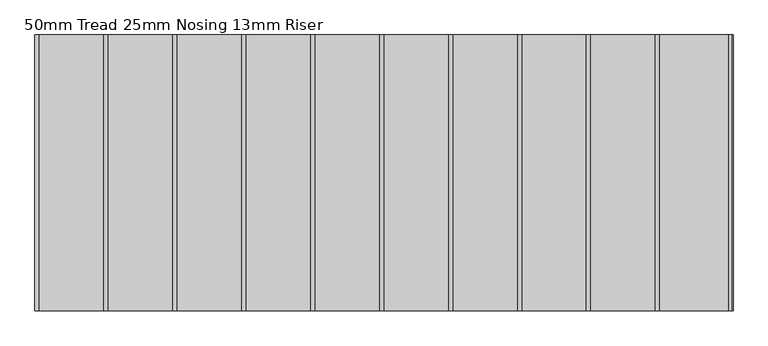
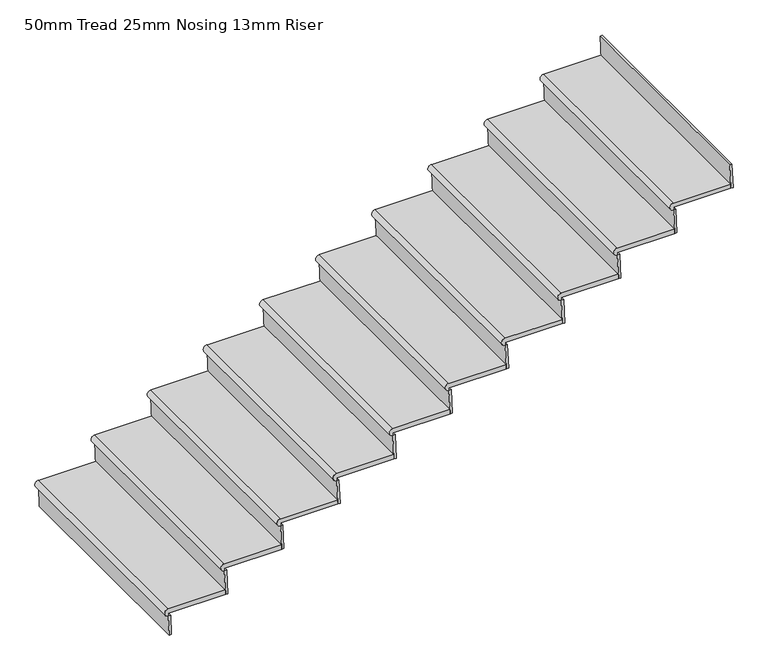
"""IFC4 building model written with IfcOpenShell, lengths in millimetres: stair flight geometry, 50mm Tread 25mm Nosing 13mm Riser."""

from ifc_helpers import new_model, si_unit, frame, origin, place, context, project, spatial, circle_curve, faceted_brep, source, transform, mapped, element, save
from ifc_brep_helpers import plane_surface, cylinder_surface, advanced_brep


def stair_flight_50mm_tread_25mm_nosing_13mm_riser_a6b179a3(model_context):
    return source(origin(), model_context, "Body", "SolidModel", [
        advanced_brep(
        [(7179.2583908, 2407.2640673, 152.4), (7180.388284, 2407.2640673, 127.0), (7180.388284, 3626.4640673, 127.0), (7179.2583908, 3626.4640673, 152.4), (6869.4583908, 3626.4640673, 152.4), (6869.4583908, 2407.2640673, 152.4), (6869.4583908, 2407.2640673, 127.0), (6869.4583908, 3626.4640673, 127.0), (6869.4583908, 3626.4640673, 112.4), (6869.4583908, 2407.2640673, 112.4)],
        [
            (0, 1),
            (1, 2),
            (2, 3),
            (3, 0),
            (3, 4),
            (4, 5),
            (5, 0),
            (1, 6),
            (6, 7),
            (7, 2),
            (7, 8),
            (8, 4, circle_curve(frame((6869.4583908, 3626.4640673, 132.4), z_axis=(0.0, 1.0, 0.0), x_axis=(1.0, 0.0, 0.0)), 20.0)),
            (5, 9, circle_curve(frame((6869.4583908, 2407.2640673, 132.4), z_axis=(0.0, -1.0, 0.0), x_axis=(1.0, 0.0, 0.0)), 20.0)),
            (9, 6),
            (8, 9),
        ],
        [
            plane_surface(frame((7180.388284, 2407.2640673, 127.0), z_axis=(0.9990120534936051, 0.0, 0.04444003796679731), x_axis=(0.0, 1.0, 0.0))),
            plane_surface(frame((6849.4583908, 3626.4640673, 152.4), z_axis=(0.0, 0.0, 1.0), x_axis=(-1.0, 0.0, 0.0))),
            plane_surface(frame((6849.4583908, 3626.4640673, 127.0), z_axis=(0.0, 0.0, -1.0), x_axis=(1.0, 0.0, 0.0))),
            plane_surface(frame((7179.2583908, 3626.4640673, 152.4), z_axis=(0.0, 1.0, 0.0), x_axis=(0.0, 0.0, -1.0))),
            plane_surface(frame((6869.4583908, 2407.2640673, 152.4), z_axis=(0.0, -1.0, 0.0), x_axis=(0.0, 0.0, -1.0))),
            cylinder_surface(frame((6869.4583908, 2407.2640673, 132.4), z_axis=(0.0, -1.0, 0.0), x_axis=(1.0, 0.0, 0.0)), 20.0),
            plane_surface(frame((6869.4583908, 2407.2640673, 112.4), z_axis=(1.0, 0.0, 0.0), x_axis=(0.0, 1.0, 0.0))),
        ],
        [
            (0, [[1, 2, 3, 4]]),
            (1, [[5, 6, 7, -4]]),
            (2, [[-2, 8, 9, 10]]),
            (3, [[-5, -3, -10, 11, 12]]),
            (4, [[-7, 13, 14, -8, -1]]),
            (5, [[-13, -6, -12, 15]]),
            (6, [[-15, -11, -9, -14]]),
        ],
    ),
        faceted_brep([(6869.4583908, 2407.2640673, 112.4), (6874.4583908, 2407.2640673, 0.0), (6886.9707523, 2407.2640673, 0.0), (6881.9707523, 2407.2640673, 112.4), (6869.4583908, 3626.4640673, 112.4), (6881.9707523, 3626.4640673, 112.4), (6886.9707523, 3626.4640673, 0.0), (6874.4583908, 3626.4640673, 0.0)], [[[0, 1, 2, 3]], [[4, 5, 6, 7]], [[1, 0, 4, 7]], [[2, 1, 7, 6]], [[3, 2, 6, 5]], [[0, 3, 5, 4]]]),
        faceted_brep([(7174.2583908, 2407.2640673, 264.8), (7180.388284, 2407.2640673, 127.0), (7192.9006455, 2407.2640673, 127.0), (7186.7707523, 2407.2640673, 264.8), (7174.2583908, 3626.4640673, 264.8), (7186.7707523, 3626.4640673, 264.8), (7192.9006455, 3626.4640673, 127.0), (7180.388284, 3626.4640673, 127.0)], [[[0, 1, 2, 3]], [[4, 5, 6, 7]], [[1, 0, 4, 7]], [[2, 1, 7, 6]], [[3, 2, 6, 5]], [[0, 3, 5, 4]]]),
        advanced_brep(
        [(7484.0583908, 3626.4640673, 304.8), (7174.2583908, 3626.4640673, 304.8), (7174.2583908, 2407.2640673, 304.8), (7484.0583908, 2407.2640673, 304.8), (7485.188284, 3626.4640673, 279.4), (7485.188284, 2407.2640673, 279.4), (7174.2583908, 2407.2640673, 279.4), (7174.2583908, 3626.4640673, 279.4), (7174.2583908, 3626.4640673, 264.8), (7174.2583908, 2407.2640673, 264.8)],
        [
            (0, 1),
            (1, 2),
            (2, 3),
            (3, 0),
            (4, 5),
            (5, 6),
            (6, 7),
            (7, 4),
            (0, 4),
            (7, 8),
            (8, 1, circle_curve(frame((7174.2583908, 3626.4640673, 284.8), z_axis=(0.0, 1.0, 0.0), x_axis=(1.0, 0.0, 0.0)), 20.0)),
            (2, 9, circle_curve(frame((7174.2583908, 2407.2640673, 284.8), z_axis=(0.0, -1.0, 0.0), x_axis=(1.0, 0.0, 0.0)), 20.0)),
            (9, 6),
            (5, 3),
            (8, 9),
        ],
        [
            plane_surface(frame((6849.4583908, 3626.4640673, 304.8), z_axis=(0.0, 0.0, 1.0), x_axis=(-1.0, 0.0, 0.0))),
            plane_surface(frame((6849.4583908, 3626.4640673, 279.4), z_axis=(0.0, 0.0, -1.0), x_axis=(1.0, 0.0, 0.0))),
            plane_surface(frame((7484.0583908, 3626.4640673, 304.8), z_axis=(0.0, 1.0, 0.0), x_axis=(0.0, 0.0, -1.0))),
            plane_surface(frame((7174.2583908, 2407.2640673, 304.8), z_axis=(0.0, -1.0, 0.0), x_axis=(0.0, 0.0, -1.0))),
            plane_surface(frame((7485.188284, 2407.2640673, 279.4), z_axis=(0.9990120534936051, 0.0, 0.04444003796679731), x_axis=(0.0, 1.0, 0.0))),
            cylinder_surface(frame((7174.2583908, 2407.2640673, 284.8), z_axis=(0.0, -1.0, 0.0), x_axis=(1.0, 0.0, 0.0)), 20.0),
            plane_surface(frame((7174.2583908, 2407.2640673, 264.8), z_axis=(1.0, 0.0, 0.0), x_axis=(0.0, 1.0, 0.0))),
        ],
        [
            (0, [[1, 2, 3, 4]]),
            (1, [[5, 6, 7, 8]]),
            (2, [[-1, 9, -8, 10, 11]]),
            (3, [[-3, 12, 13, -6, 14]]),
            (4, [[-14, -5, -9, -4]]),
            (5, [[-12, -2, -11, 15]]),
            (6, [[-15, -10, -7, -13]]),
        ],
    ),
        faceted_brep([(7479.0583908, 2407.2640673, 417.2), (7485.188284, 2407.2640673, 279.4), (7497.7006455, 2407.2640673, 279.4), (7491.5707523, 2407.2640673, 417.2), (7479.0583908, 3626.4640673, 417.2), (7491.5707523, 3626.4640673, 417.2), (7497.7006455, 3626.4640673, 279.4), (7485.188284, 3626.4640673, 279.4)], [[[0, 1, 2, 3]], [[4, 5, 6, 7]], [[1, 0, 4, 7]], [[2, 1, 7, 6]], [[3, 2, 6, 5]], [[0, 3, 5, 4]]]),
        advanced_brep(
        [(7788.8583908, 3626.4640673, 457.2), (7479.0583908, 3626.4640673, 457.2), (7479.0583908, 2407.2640673, 457.2), (7788.8583908, 2407.2640673, 457.2), (7789.988284, 3626.4640673, 431.8), (7789.988284, 2407.2640673, 431.8), (7479.0583908, 2407.2640673, 431.8), (7479.0583908, 3626.4640673, 431.8), (7479.0583908, 3626.4640673, 417.2), (7479.0583908, 2407.2640673, 417.2)],
        [
            (0, 1),
            (1, 2),
            (2, 3),
            (3, 0),
            (4, 5),
            (5, 6),
            (6, 7),
            (7, 4),
            (0, 4),
            (7, 8),
            (8, 1, circle_curve(frame((7479.0583908, 3626.4640673, 437.2), z_axis=(0.0, 1.0, 0.0), x_axis=(1.0, 0.0, 0.0)), 20.0)),
            (2, 9, circle_curve(frame((7479.0583908, 2407.2640673, 437.2), z_axis=(0.0, -1.0, 0.0), x_axis=(1.0, 0.0, 0.0)), 20.0)),
            (9, 6),
            (5, 3),
            (8, 9),
        ],
        [
            plane_surface(frame((7154.2583908, 3626.4640673, 457.2), z_axis=(0.0, 0.0, 1.0), x_axis=(-1.0, 0.0, 0.0))),
            plane_surface(frame((7154.2583908, 3626.4640673, 431.8), z_axis=(0.0, 0.0, -1.0), x_axis=(1.0, 0.0, 0.0))),
            plane_surface(frame((7788.8583908, 3626.4640673, 457.2), z_axis=(0.0, 1.0, 0.0), x_axis=(0.0, 0.0, -1.0))),
            plane_surface(frame((7479.0583908, 2407.2640673, 457.2), z_axis=(0.0, -1.0, 0.0), x_axis=(0.0, 0.0, -1.0))),
            plane_surface(frame((7789.988284, 2407.2640673, 431.8), z_axis=(0.9990120534936051, 0.0, 0.04444003796679731), x_axis=(0.0, 1.0, 0.0))),
            cylinder_surface(frame((7479.0583908, 2407.2640673, 437.2), z_axis=(0.0, -1.0, 0.0), x_axis=(1.0, 0.0, 0.0)), 20.0),
            plane_surface(frame((7479.0583908, 2407.2640673, 417.2), z_axis=(1.0, 0.0, 0.0), x_axis=(0.0, 1.0, 0.0))),
        ],
        [
            (0, [[1, 2, 3, 4]]),
            (1, [[5, 6, 7, 8]]),
            (2, [[-1, 9, -8, 10, 11]]),
            (3, [[-3, 12, 13, -6, 14]]),
            (4, [[-14, -5, -9, -4]]),
            (5, [[-12, -2, -11, 15]]),
            (6, [[-15, -10, -7, -13]]),
        ],
    ),
        faceted_brep([(7783.8583908, 2407.2640673, 569.6), (7789.988284, 2407.2640673, 431.8), (7802.5006455, 2407.2640673, 431.8), (7796.3707523, 2407.2640673, 569.6), (7783.8583908, 3626.4640673, 569.6), (7796.3707523, 3626.4640673, 569.6), (7802.5006455, 3626.4640673, 431.8), (7789.988284, 3626.4640673, 431.8)], [[[0, 1, 2, 3]], [[4, 5, 6, 7]], [[1, 0, 4, 7]], [[2, 1, 7, 6]], [[3, 2, 6, 5]], [[0, 3, 5, 4]]]),
        advanced_brep(
        [(8093.6583908, 3626.4640673, 609.6), (7783.8583908, 3626.4640673, 609.6), (7783.8583908, 2407.2640673, 609.6), (8093.6583908, 2407.2640673, 609.6), (8094.788284, 3626.4640673, 584.2), (8094.788284, 2407.2640673, 584.2), (7783.8583908, 2407.2640673, 584.2), (7783.8583908, 3626.4640673, 584.2), (7783.8583908, 3626.4640673, 569.6), (7783.8583908, 2407.2640673, 569.6)],
        [
            (0, 1),
            (1, 2),
            (2, 3),
            (3, 0),
            (4, 5),
            (5, 6),
            (6, 7),
            (7, 4),
            (0, 4),
            (7, 8),
            (8, 1, circle_curve(frame((7783.8583908, 3626.4640673, 589.6), z_axis=(0.0, 1.0, 0.0), x_axis=(1.0, 0.0, 0.0)), 20.0)),
            (2, 9, circle_curve(frame((7783.8583908, 2407.2640673, 589.6), z_axis=(0.0, -1.0, 0.0), x_axis=(1.0, 0.0, 0.0)), 20.0)),
            (9, 6),
            (5, 3),
            (8, 9),
        ],
        [
            plane_surface(frame((7459.0583908, 3626.4640673, 609.6), z_axis=(0.0, 0.0, 1.0), x_axis=(-1.0, 0.0, 0.0))),
            plane_surface(frame((7459.0583908, 3626.4640673, 584.2), z_axis=(0.0, 0.0, -1.0), x_axis=(1.0, 0.0, 0.0))),
            plane_surface(frame((8093.6583908, 3626.4640673, 609.6), z_axis=(0.0, 1.0, 0.0), x_axis=(0.0, 0.0, -1.0))),
            plane_surface(frame((7783.8583908, 2407.2640673, 609.6), z_axis=(0.0, -1.0, 0.0), x_axis=(0.0, 0.0, -1.0))),
            plane_surface(frame((8094.788284, 2407.2640673, 584.2), z_axis=(0.9990120534936051, 0.0, 0.04444003796679731), x_axis=(0.0, 1.0, 0.0))),
            cylinder_surface(frame((7783.8583908, 2407.2640673, 589.6), z_axis=(0.0, -1.0, 0.0), x_axis=(1.0, 0.0, 0.0)), 20.0),
            plane_surface(frame((7783.8583908, 2407.2640673, 569.6), z_axis=(1.0, 0.0, 0.0), x_axis=(0.0, 1.0, 0.0))),
        ],
        [
            (0, [[1, 2, 3, 4]]),
            (1, [[5, 6, 7, 8]]),
            (2, [[-1, 9, -8, 10, 11]]),
            (3, [[-3, 12, 13, -6, 14]]),
            (4, [[-14, -5, -9, -4]]),
            (5, [[-12, -2, -11, 15]]),
            (6, [[-15, -10, -7, -13]]),
        ],
    ),
        faceted_brep([(8088.6583908, 2407.2640673, 722.0), (8094.788284, 2407.2640673, 584.2), (8107.3006455, 2407.2640673, 584.2), (8101.1707523, 2407.2640673, 722.0), (8088.6583908, 3626.4640673, 722.0), (8101.1707523, 3626.4640673, 722.0), (8107.3006455, 3626.4640673, 584.2), (8094.788284, 3626.4640673, 584.2)], [[[0, 1, 2, 3]], [[4, 5, 6, 7]], [[1, 0, 4, 7]], [[2, 1, 7, 6]], [[3, 2, 6, 5]], [[0, 3, 5, 4]]]),
        advanced_brep(
        [(8398.4583908, 3626.4640673, 762.0), (8088.6583908, 3626.4640673, 762.0), (8088.6583908, 2407.2640673, 762.0), (8398.4583908, 2407.2640673, 762.0), (8399.588284, 3626.4640673, 736.6), (8399.588284, 2407.2640673, 736.6), (8088.6583908, 2407.2640673, 736.6), (8088.6583908, 3626.4640673, 736.6), (8088.6583908, 3626.4640673, 722.0), (8088.6583908, 2407.2640673, 722.0)],
        [
            (0, 1),
            (1, 2),
            (2, 3),
            (3, 0),
            (4, 5),
            (5, 6),
            (6, 7),
            (7, 4),
            (0, 4),
            (7, 8),
            (8, 1, circle_curve(frame((8088.6583908, 3626.4640673, 742.0), z_axis=(0.0, 1.0, 0.0), x_axis=(1.0, 0.0, 0.0)), 20.0)),
            (2, 9, circle_curve(frame((8088.6583908, 2407.2640673, 742.0), z_axis=(0.0, -1.0, 0.0), x_axis=(1.0, 0.0, 0.0)), 20.0)),
            (9, 6),
            (5, 3),
            (8, 9),
        ],
        [
            plane_surface(frame((7763.8583908, 3626.4640673, 762.0), z_axis=(0.0, 0.0, 1.0), x_axis=(-1.0, 0.0, 0.0))),
            plane_surface(frame((7763.8583908, 3626.4640673, 736.6), z_axis=(0.0, 0.0, -1.0), x_axis=(1.0, 0.0, 0.0))),
            plane_surface(frame((8398.4583908, 3626.4640673, 762.0), z_axis=(0.0, 1.0, 0.0), x_axis=(0.0, 0.0, -1.0))),
            plane_surface(frame((8088.6583908, 2407.2640673, 762.0), z_axis=(0.0, -1.0, 0.0), x_axis=(0.0, 0.0, -1.0))),
            plane_surface(frame((8399.588284, 2407.2640673, 736.6), z_axis=(0.9990120534936051, 0.0, 0.04444003796679731), x_axis=(0.0, 1.0, 0.0))),
            cylinder_surface(frame((8088.6583908, 2407.2640673, 742.0), z_axis=(0.0, -1.0, 0.0), x_axis=(1.0, 0.0, 0.0)), 20.0),
            plane_surface(frame((8088.6583908, 2407.2640673, 722.0), z_axis=(1.0, 0.0, 0.0), x_axis=(0.0, 1.0, 0.0))),
        ],
        [
            (0, [[1, 2, 3, 4]]),
            (1, [[5, 6, 7, 8]]),
            (2, [[-1, 9, -8, 10, 11]]),
            (3, [[-3, 12, 13, -6, 14]]),
            (4, [[-14, -5, -9, -4]]),
            (5, [[-12, -2, -11, 15]]),
            (6, [[-15, -10, -7, -13]]),
        ],
    ),
        faceted_brep([(8393.4583908, 2407.2640673, 874.4), (8399.588284, 2407.2640673, 736.6), (8412.1006455, 2407.2640673, 736.6), (8405.9707523, 2407.2640673, 874.4), (8393.4583908, 3626.4640673, 874.4), (8405.9707523, 3626.4640673, 874.4), (8412.1006455, 3626.4640673, 736.6), (8399.588284, 3626.4640673, 736.6)], [[[0, 1, 2, 3]], [[4, 5, 6, 7]], [[1, 0, 4, 7]], [[2, 1, 7, 6]], [[3, 2, 6, 5]], [[0, 3, 5, 4]]]),
        advanced_brep(
        [(8703.2583908, 3626.4640673, 914.4), (8393.4583908, 3626.4640673, 914.4), (8393.4583908, 2407.2640673, 914.4), (8703.2583908, 2407.2640673, 914.4), (8704.388284, 3626.4640673, 889.0), (8704.388284, 2407.2640673, 889.0), (8393.4583908, 2407.2640673, 889.0), (8393.4583908, 3626.4640673, 889.0), (8393.4583908, 3626.4640673, 874.4), (8393.4583908, 2407.2640673, 874.4)],
        [
            (0, 1),
            (1, 2),
            (2, 3),
            (3, 0),
            (4, 5),
            (5, 6),
            (6, 7),
            (7, 4),
            (0, 4),
            (7, 8),
            (8, 1, circle_curve(frame((8393.4583908, 3626.4640673, 894.4), z_axis=(0.0, 1.0, 0.0), x_axis=(1.0, 0.0, 0.0)), 20.0)),
            (2, 9, circle_curve(frame((8393.4583908, 2407.2640673, 894.4), z_axis=(0.0, -1.0, 0.0), x_axis=(1.0, 0.0, 0.0)), 20.0)),
            (9, 6),
            (5, 3),
            (8, 9),
        ],
        [
            plane_surface(frame((8068.6583908, 3626.4640673, 914.4), z_axis=(0.0, 0.0, 1.0), x_axis=(-1.0, 0.0, 0.0))),
            plane_surface(frame((8068.6583908, 3626.4640673, 889.0), z_axis=(0.0, 0.0, -1.0), x_axis=(1.0, 0.0, 0.0))),
            plane_surface(frame((8703.2583908, 3626.4640673, 914.4), z_axis=(0.0, 1.0, 0.0), x_axis=(0.0, 0.0, -1.0))),
            plane_surface(frame((8393.4583908, 2407.2640673, 914.4), z_axis=(0.0, -1.0, 0.0), x_axis=(0.0, 0.0, -1.0))),
            plane_surface(frame((8704.388284, 2407.2640673, 889.0), z_axis=(0.9990120534936051, 0.0, 0.04444003796679731), x_axis=(0.0, 1.0, 0.0))),
            cylinder_surface(frame((8393.4583908, 2407.2640673, 894.4), z_axis=(0.0, -1.0, 0.0), x_axis=(1.0, 0.0, 0.0)), 20.0),
            plane_surface(frame((8393.4583908, 2407.2640673, 874.4), z_axis=(1.0, 0.0, 0.0), x_axis=(0.0, 1.0, 0.0))),
        ],
        [
            (0, [[1, 2, 3, 4]]),
            (1, [[5, 6, 7, 8]]),
            (2, [[-1, 9, -8, 10, 11]]),
            (3, [[-3, 12, 13, -6, 14]]),
            (4, [[-14, -5, -9, -4]]),
            (5, [[-12, -2, -11, 15]]),
            (6, [[-15, -10, -7, -13]]),
        ],
    ),
        faceted_brep([(8698.2583908, 2407.2640673, 1026.8), (8704.388284, 2407.2640673, 889.0), (8716.9006455, 2407.2640673, 889.0), (8710.7707523, 2407.2640673, 1026.8), (8698.2583908, 3626.4640673, 1026.8), (8710.7707523, 3626.4640673, 1026.8), (8716.9006455, 3626.4640673, 889.0), (8704.388284, 3626.4640673, 889.0)], [[[0, 1, 2, 3]], [[4, 5, 6, 7]], [[1, 0, 4, 7]], [[2, 1, 7, 6]], [[3, 2, 6, 5]], [[0, 3, 5, 4]]]),
        advanced_brep(
        [(9008.0583908, 3626.4640673, 1066.8), (8698.2583908, 3626.4640673, 1066.8), (8698.2583908, 2407.2640673, 1066.8), (9008.0583908, 2407.2640673, 1066.8), (9009.188284, 3626.4640673, 1041.4), (9009.188284, 2407.2640673, 1041.4), (8698.2583908, 2407.2640673, 1041.4), (8698.2583908, 3626.4640673, 1041.4), (8698.2583908, 3626.4640673, 1026.8), (8698.2583908, 2407.2640673, 1026.8)],
        [
            (0, 1),
            (1, 2),
            (2, 3),
            (3, 0),
            (4, 5),
            (5, 6),
            (6, 7),
            (7, 4),
            (0, 4),
            (7, 8),
            (8, 1, circle_curve(frame((8698.2583908, 3626.4640673, 1046.8), z_axis=(0.0, 1.0, 0.0), x_axis=(1.0, 0.0, 0.0)), 20.0)),
            (2, 9, circle_curve(frame((8698.2583908, 2407.2640673, 1046.8), z_axis=(0.0, -1.0, 0.0), x_axis=(1.0, 0.0, 0.0)), 20.0)),
            (9, 6),
            (5, 3),
            (8, 9),
        ],
        [
            plane_surface(frame((8373.4583908, 3626.4640673, 1066.8), z_axis=(0.0, 0.0, 1.0), x_axis=(-1.0, 0.0, 0.0))),
            plane_surface(frame((8373.4583908, 3626.4640673, 1041.4), z_axis=(0.0, 0.0, -1.0), x_axis=(1.0, 0.0, 0.0))),
            plane_surface(frame((9008.0583908, 3626.4640673, 1066.8), z_axis=(0.0, 1.0, 0.0), x_axis=(0.0, 0.0, -1.0))),
            plane_surface(frame((8698.2583908, 2407.2640673, 1066.8), z_axis=(0.0, -1.0, 0.0), x_axis=(0.0, 0.0, -1.0))),
            plane_surface(frame((9009.188284, 2407.2640673, 1041.4), z_axis=(0.9990120534936051, 0.0, 0.04444003796679731), x_axis=(0.0, 1.0, 0.0))),
            cylinder_surface(frame((8698.2583908, 2407.2640673, 1046.8), z_axis=(0.0, -1.0, 0.0), x_axis=(1.0, 0.0, 0.0)), 20.0),
            plane_surface(frame((8698.2583908, 2407.2640673, 1026.8), z_axis=(1.0, 0.0, 0.0), x_axis=(0.0, 1.0, 0.0))),
        ],
        [
            (0, [[1, 2, 3, 4]]),
            (1, [[5, 6, 7, 8]]),
            (2, [[-1, 9, -8, 10, 11]]),
            (3, [[-3, 12, 13, -6, 14]]),
            (4, [[-14, -5, -9, -4]]),
            (5, [[-12, -2, -11, 15]]),
            (6, [[-15, -10, -7, -13]]),
        ],
    ),
        faceted_brep([(9003.0583908, 2407.2640673, 1179.2), (9009.188284, 2407.2640673, 1041.4), (9021.7006455, 2407.2640673, 1041.4), (9015.5707523, 2407.2640673, 1179.2), (9003.0583908, 3626.4640673, 1179.2), (9015.5707523, 3626.4640673, 1179.2), (9021.7006455, 3626.4640673, 1041.4), (9009.188284, 3626.4640673, 1041.4)], [[[0, 1, 2, 3]], [[4, 5, 6, 7]], [[1, 0, 4, 7]], [[2, 1, 7, 6]], [[3, 2, 6, 5]], [[0, 3, 5, 4]]]),
        advanced_brep(
        [(9312.8583908, 3626.4640673, 1219.2), (9003.0583908, 3626.4640673, 1219.2), (9003.0583908, 2407.2640673, 1219.2), (9312.8583908, 2407.2640673, 1219.2), (9313.988284, 3626.4640673, 1193.8), (9313.988284, 2407.2640673, 1193.8), (9003.0583908, 2407.2640673, 1193.8), (9003.0583908, 3626.4640673, 1193.8), (9003.0583908, 3626.4640673, 1179.2), (9003.0583908, 2407.2640673, 1179.2)],
        [
            (0, 1),
            (1, 2),
            (2, 3),
            (3, 0),
            (4, 5),
            (5, 6),
            (6, 7),
            (7, 4),
            (0, 4),
            (7, 8),
            (8, 1, circle_curve(frame((9003.0583908, 3626.4640673, 1199.2), z_axis=(0.0, 1.0, 0.0), x_axis=(1.0, 0.0, 0.0)), 20.0)),
            (2, 9, circle_curve(frame((9003.0583908, 2407.2640673, 1199.2), z_axis=(0.0, -1.0, 0.0), x_axis=(1.0, 0.0, 0.0)), 20.0)),
            (9, 6),
            (5, 3),
            (8, 9),
        ],
        [
            plane_surface(frame((8678.2583908, 3626.4640673, 1219.2), z_axis=(0.0, 0.0, 1.0), x_axis=(-1.0, 0.0, 0.0))),
            plane_surface(frame((8678.2583908, 3626.4640673, 1193.8), z_axis=(0.0, 0.0, -1.0), x_axis=(1.0, 0.0, 0.0))),
            plane_surface(frame((9312.8583908, 3626.4640673, 1219.2), z_axis=(0.0, 1.0, 0.0), x_axis=(0.0, 0.0, -1.0))),
            plane_surface(frame((9003.0583908, 2407.2640673, 1219.2), z_axis=(0.0, -1.0, 0.0), x_axis=(0.0, 0.0, -1.0))),
            plane_surface(frame((9313.988284, 2407.2640673, 1193.8), z_axis=(0.9990120534936051, 0.0, 0.04444003796679731), x_axis=(0.0, 1.0, 0.0))),
            cylinder_surface(frame((9003.0583908, 2407.2640673, 1199.2), z_axis=(0.0, -1.0, 0.0), x_axis=(1.0, 0.0, 0.0)), 20.0),
            plane_surface(frame((9003.0583908, 2407.2640673, 1179.2), z_axis=(1.0, 0.0, 0.0), x_axis=(0.0, 1.0, 0.0))),
        ],
        [
            (0, [[1, 2, 3, 4]]),
            (1, [[5, 6, 7, 8]]),
            (2, [[-1, 9, -8, 10, 11]]),
            (3, [[-3, 12, 13, -6, 14]]),
            (4, [[-14, -5, -9, -4]]),
            (5, [[-12, -2, -11, 15]]),
            (6, [[-15, -10, -7, -13]]),
        ],
    ),
        faceted_brep([(9307.8583908, 2407.2640673, 1331.6), (9313.988284, 2407.2640673, 1193.8), (9326.5006455, 2407.2640673, 1193.8), (9320.3707523, 2407.2640673, 1331.6), (9307.8583908, 3626.4640673, 1331.6), (9320.3707523, 3626.4640673, 1331.6), (9326.5006455, 3626.4640673, 1193.8), (9313.988284, 3626.4640673, 1193.8)], [[[0, 1, 2, 3]], [[4, 5, 6, 7]], [[1, 0, 4, 7]], [[2, 1, 7, 6]], [[3, 2, 6, 5]], [[0, 3, 5, 4]]]),
        advanced_brep(
        [(9617.6583908, 3626.4640673, 1371.6), (9307.8583908, 3626.4640673, 1371.6), (9307.8583908, 2407.2640673, 1371.6), (9617.6583908, 2407.2640673, 1371.6), (9618.788284, 3626.4640673, 1346.2), (9618.788284, 2407.2640673, 1346.2), (9307.8583908, 2407.2640673, 1346.2), (9307.8583908, 3626.4640673, 1346.2), (9307.8583908, 3626.4640673, 1331.6), (9307.8583908, 2407.2640673, 1331.6)],
        [
            (0, 1),
            (1, 2),
            (2, 3),
            (3, 0),
            (4, 5),
            (5, 6),
            (6, 7),
            (7, 4),
            (0, 4),
            (7, 8),
            (8, 1, circle_curve(frame((9307.8583908, 3626.4640673, 1351.6), z_axis=(0.0, 1.0, 0.0), x_axis=(1.0, 0.0, 0.0)), 20.0)),
            (2, 9, circle_curve(frame((9307.8583908, 2407.2640673, 1351.6), z_axis=(0.0, -1.0, 0.0), x_axis=(1.0, 0.0, 0.0)), 20.0)),
            (9, 6),
            (5, 3),
            (8, 9),
        ],
        [
            plane_surface(frame((8983.0583908, 3626.4640673, 1371.6), z_axis=(0.0, 0.0, 1.0), x_axis=(-1.0, 0.0, 0.0))),
            plane_surface(frame((8983.0583908, 3626.4640673, 1346.2), z_axis=(0.0, 0.0, -1.0), x_axis=(1.0, 0.0, 0.0))),
            plane_surface(frame((9617.6583908, 3626.4640673, 1371.6), z_axis=(0.0, 1.0, 0.0), x_axis=(0.0, 0.0, -1.0))),
            plane_surface(frame((9307.8583908, 2407.2640673, 1371.6), z_axis=(0.0, -1.0, 0.0), x_axis=(0.0, 0.0, -1.0))),
            plane_surface(frame((9618.788284, 2407.2640673, 1346.2), z_axis=(0.9990120534936051, 0.0, 0.04444003796679731), x_axis=(0.0, 1.0, 0.0))),
            cylinder_surface(frame((9307.8583908, 2407.2640673, 1351.6), z_axis=(0.0, -1.0, 0.0), x_axis=(1.0, 0.0, 0.0)), 20.0),
            plane_surface(frame((9307.8583908, 2407.2640673, 1331.6), z_axis=(1.0, 0.0, 0.0), x_axis=(0.0, 1.0, 0.0))),
        ],
        [
            (0, [[1, 2, 3, 4]]),
            (1, [[5, 6, 7, 8]]),
            (2, [[-1, 9, -8, 10, 11]]),
            (3, [[-3, 12, 13, -6, 14]]),
            (4, [[-14, -5, -9, -4]]),
            (5, [[-12, -2, -11, 15]]),
            (6, [[-15, -10, -7, -13]]),
        ],
    ),
        faceted_brep([(9917.4583908, 2407.2640673, 1636.4), (9923.588284, 2407.2640673, 1498.6), (9936.1006455, 2407.2640673, 1498.6), (9929.9707523, 2407.2640673, 1636.4), (9917.4583908, 3626.4640673, 1636.4), (9929.9707523, 3626.4640673, 1636.4), (9936.1006455, 3626.4640673, 1498.6), (9923.588284, 3626.4640673, 1498.6)], [[[0, 1, 2, 3]], [[4, 5, 6, 7]], [[1, 0, 4, 7]], [[2, 1, 7, 6]], [[3, 2, 6, 5]], [[0, 3, 5, 4]]]),
        faceted_brep([(9612.6583908, 2407.2640673, 1484.0), (9618.788284, 2407.2640673, 1346.2), (9631.3006455, 2407.2640673, 1346.2), (9625.1707523, 2407.2640673, 1484.0), (9612.6583908, 3626.4640673, 1484.0), (9625.1707523, 3626.4640673, 1484.0), (9631.3006455, 3626.4640673, 1346.2), (9618.788284, 3626.4640673, 1346.2)], [[[0, 1, 2, 3]], [[4, 5, 6, 7]], [[1, 0, 4, 7]], [[2, 1, 7, 6]], [[3, 2, 6, 5]], [[0, 3, 5, 4]]]),
        advanced_brep(
        [(9922.4583908, 3626.4640673, 1524.0), (9897.4583908, 3626.4640673, 1524.0), (9612.6583908, 3626.4640673, 1524.0), (9612.6583908, 2407.2640673, 1524.0), (9922.4583908, 2407.2640673, 1524.0), (9612.6583908, 3626.4640673, 1498.6), (9897.4583908, 3626.4640673, 1498.6), (9923.588284, 3626.4640673, 1498.6), (9923.588284, 2407.2640673, 1498.6), (9612.6583908, 2407.2640673, 1498.6), (9612.6583908, 3626.4640673, 1484.0), (9612.6583908, 2407.2640673, 1484.0)],
        [
            (0, 1),
            (1, 2),
            (2, 3),
            (3, 4),
            (4, 0),
            (5, 6),
            (6, 7),
            (7, 8),
            (8, 9),
            (9, 5),
            (0, 7),
            (6, 1),
            (5, 10),
            (10, 2, circle_curve(frame((9612.6583908, 3626.4640673, 1504.0), z_axis=(0.0, 1.0, 0.0), x_axis=(1.0, 0.0, 0.0)), 20.0)),
            (3, 11, circle_curve(frame((9612.6583908, 2407.2640673, 1504.0), z_axis=(0.0, -1.0, 0.0), x_axis=(1.0, 0.0, 0.0)), 20.0)),
            (11, 9),
            (8, 4),
            (10, 11),
        ],
        [
            plane_surface(frame((9897.4583908, 3626.4640673, 1524.0), z_axis=(0.0, 0.0, 1.0), x_axis=(-1.0, 0.0, 0.0))),
            plane_surface(frame((9897.4583908, 3626.4640673, 1498.6), z_axis=(0.0, 0.0, -1.0), x_axis=(1.0, 0.0, 0.0))),
            plane_surface(frame((9922.4583908, 3626.4640673, 1524.0), z_axis=(0.0, 1.0, 0.0), x_axis=(0.0, 0.0, -1.0))),
            plane_surface(frame((9897.4583908, 3626.4640673, 1524.0), z_axis=(0.0, 1.0, 0.0), x_axis=(0.0, 0.0, -1.0))),
            plane_surface(frame((9612.6583908, 2407.2640673, 1524.0), z_axis=(0.0, -1.0, 0.0), x_axis=(0.0, 0.0, -1.0))),
            plane_surface(frame((9923.588284, 2407.2640673, 1498.6), z_axis=(0.9990120534936051, 0.0, 0.04444003796679731), x_axis=(0.0, 1.0, 0.0))),
            cylinder_surface(frame((9612.6583908, 2407.2640673, 1504.0), z_axis=(0.0, -1.0, 0.0), x_axis=(1.0, 0.0, 0.0)), 20.0),
            plane_surface(frame((9612.6583908, 2407.2640673, 1484.0), z_axis=(1.0, 0.0, 0.0), x_axis=(0.0, 1.0, 0.0))),
        ],
        [
            (0, [[1, 2, 3, 4, 5]]),
            (1, [[6, 7, 8, 9, 10]]),
            (2, [[-1, 11, -7, 12]]),
            (3, [[-2, -12, -6, 13, 14]]),
            (4, [[-4, 15, 16, -9, 17]]),
            (5, [[-17, -8, -11, -5]]),
            (6, [[-15, -3, -14, 18]]),
            (7, [[-18, -13, -10, -16]]),
        ],
    ),
    ])


if __name__ == "__main__":
    model = new_model("IFC4")
    model_context = context("Model", 3, world=origin())
    ifc_project = project(units=[si_unit("LENGTHUNIT", "METRE", prefix="MILLI")], contexts=[model_context])
    site = spatial("IfcSite", under=ifc_project)
    building = spatial("IfcBuilding", under=site)
    placement = place(None, origin())
    stair_flight_50mm_tread_25mm_nosing_13mm_riser_shape = stair_flight_50mm_tread_25mm_nosing_13mm_riser_a6b179a3(model_context)
    element("IfcStairFlight", 1, ObjectType="50mm Tread 25mm Nosing 13mm Riser", at=placement, inside=building, context=model_context, shape_type="MappedRepresentation", body=[
        mapped(stair_flight_50mm_tread_25mm_nosing_13mm_riser_shape, transform((0.0, 0.0, 0.0), x_axis=(1.0, 0.0, 0.0), y_axis=(0.0, 1.0, 0.0), z_axis=(0.0, 0.0, 1.0))),
    ])
    save(model, "model.ifc")
